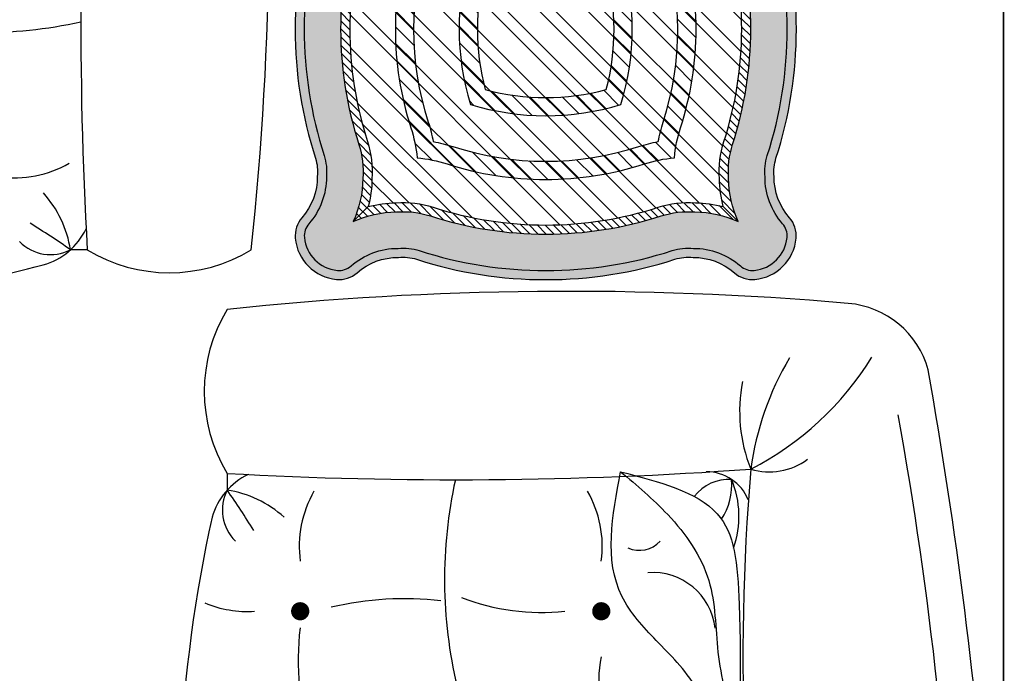
# Model space of a CAD drawing. Units: inches. Extents: x 844 to 2234, y 346 to 1084.
# Tile 41 of 93: x 1266.41 to 1283.63, y 707.78 to 719.22. Entities that reach past the tile are written whole.
import ezdxf

# ---------------------------------------------------------------- set-up
doc = ezdxf.new("R2010")
doc.units = ezdxf.units.IN
doc.header["$MEASUREMENT"] = 0
doc.layers.add('A-WALL', color=7, linetype='Continuous', lineweight=35)
doc.layers.add('furniture', color=8, linetype='Continuous', lineweight=18)
for name, color, linetype in [('RA-AP-01$0$FURN', 3, 'Continuous'), ('RA-AP-01$0$steel', 193, 'Continuous'), ('RA-AP-01$0$WOOD', 64, 'Continuous')]:
    doc.layers.add(name, color=color, linetype=linetype)
pattern_1 = [(45, (0, 1.362436106329781), (-0.0088388347648318, 0.0088388347648318), [])]
pattern_2 = [(45, (0, 1.362436106329781), (-0.0044194173824159, 0.0044194173824159), [])]

# ---------------------------------------------------------------- blocks, each defined once
blk = doc.blocks.new('A$C2FCF5309')
at = {"layer": 'RA-AP-01$0$FURN'}
h = blk.add_hatch(dxfattribs=at)
h.set_pattern_fill('ANSI31', color=256, scale=0.1, style=0)
h.set_pattern_definition(pattern_1)
h.paths.add_polyline_path([(5.038683893313746, -5.169250834004607, -0.1583983521602212), (5.038683893312098, -5.373464580902012, 0.0306258898943267), (5.033304057242972, -5.394827569605182, 0.0306258898948892), (5.01194106853941, -5.40020740567441, -0.1028142994996694), (4.878286182323899, -5.414871334512708), (4.863600873530158, -5.43331743520547, 0.1120482678681049), (5.018059823131753, -5.419248541734471, -0.052642197802937), (5.050972078299936, -5.412495590662115, -0.0526421977994963), (5.057725029371615, -5.379583335496025, 0.1583028414702701), (5.057725029372958, -5.163132079409654, -0.052642197806903), (5.050972078299777, -5.130219824239078, -0.0526421977995126), (5.018059823133679, -5.123466873167369, 0.0215995840215353), (4.988903013548211, -5.115372132362452), (4.975007495303644, -5.132826183367946, -0.0289147572844802), (5.011941068537408, -5.142508009226167, 0.0306258898976746), (5.033304057242868, -5.147887845296027, 0.0306258899022411)])
h.paths.add_polyline_path([(4.975007495303645, -5.132826183367946), (4.988903013548211, -5.115372132362452, 0.1362374241599938), (4.801608567045604, -5.12346687316654, -0.0526421978036853), (4.768696311876971, -5.130219824239102, -0.05264219780204), (4.761943360804856, -5.163132079406747, 0.1583028414743723), (4.761943360806116, -5.379583335498449, -0.0526421977955461), (4.768696311877141, -5.412495590662114, -0.0526421978073986), (4.801608567048022, -5.419248541735437, 0.0454484293938888), (4.863600873530158, -5.43331743520547), (4.878286182323899, -5.414871334512708, -0.0546933379798044), (4.80772732164382, -5.40020740567649, 0.030625889903973), (4.786364332934043, -5.394827569605216, 0.0306258898932853), (4.780984496865101, -5.373464580902791, -0.1583983521638281), (4.780984496864308, -5.169250834000963, 0.03062588989692), (4.786364332933943, -5.147887845296004, 0.0306258898946324), (4.807727321637318, -5.142508009226805, -0.1288932573266927)])
h.paths.add_polyline_path([(4.843422214712861, -5.204945727074827, -0.0783685831716868), (4.924134454130224, -5.196727409635105), (4.939146578618322, -5.177870798323143, 0.1012675676854134), (4.827248748758957, -5.188772261120899, 0.1253648873081696), (4.820394258584192, -5.327034652050361), (4.837127701354095, -5.306015906404253, -0.0981593964869636)], flags=17)
h.paths.add_polyline_path([(4.843422214712824, -5.337769687826355, -0.0311091841722656), (4.837127701354095, -5.306015906404253), (4.820394258584193, -5.32703465205036, 0.0247727657431944), (4.827248748758908, -5.353943153780261, 0.0812754385032542), (4.916962478476905, -5.36629034358622), (4.933684093813825, -5.345286454285511, -0.0876255421014372)], flags=17)
h.paths.add_polyline_path([(4.992419641418037, -5.353943153780226, 0.1506053783834298), (4.992419641417933, -5.188772261120954, 0.0485966419124224), (4.939146578618321, -5.177870798323143), (4.924134454130224, -5.196727409635105, -0.0507799419579301), (4.976246175464031, -5.204945727074882, -0.1296645318906876), (4.97624617546411, -5.337769687826316, -0.0415667119298777), (4.933684093813825, -5.345286454285511), (4.916962478476905, -5.36629034358622, 0.0684915676023693)], flags=17)
h = blk.add_hatch(dxfattribs=at)
h.set_pattern_fill('ANSI31', color=256, scale=0.1, style=0)
h.set_pattern_definition(pattern_1)
h.paths.add_polyline_path([(5.038683893313746, -5.169250834004607, -0.1583983521602212), (5.038683893312098, -5.373464580902012, 0.0306258898943267), (5.033304057242972, -5.394827569605182, 0.0306258898948892), (5.01194106853941, -5.40020740567441, -0.1028142994996694), (4.878286182323899, -5.414871334512708), (4.863600873530158, -5.43331743520547, 0.1120482678681049), (5.018059823131753, -5.419248541734471, -0.052642197802937), (5.050972078299936, -5.412495590662115, -0.0526421977994963), (5.057725029371615, -5.379583335496025, 0.1583028414702701), (5.057725029372958, -5.163132079409654, -0.052642197806903), (5.050972078299777, -5.130219824239078, -0.0526421977995126), (5.018059823133679, -5.123466873167369, 0.0215995840215353), (4.988903013548211, -5.115372132362452), (4.975007495303644, -5.132826183367946, -0.0289147572844802), (5.011941068537408, -5.142508009226167, 0.0306258898976746), (5.033304057242868, -5.147887845296027, 0.0306258899022411)])
h.paths.add_polyline_path([(4.975007495303645, -5.132826183367946), (4.988903013548211, -5.115372132362452, 0.1362374241599938), (4.801608567045604, -5.12346687316654, -0.0526421978036853), (4.768696311876971, -5.130219824239102, -0.05264219780204), (4.761943360804856, -5.163132079406747, 0.1583028414743723), (4.761943360806116, -5.379583335498449, -0.0526421977955461), (4.768696311877141, -5.412495590662114, -0.0526421978073986), (4.801608567048022, -5.419248541735437, 0.0454484293938888), (4.863600873530158, -5.43331743520547), (4.878286182323899, -5.414871334512708, -0.0546933379798044), (4.80772732164382, -5.40020740567649, 0.030625889903973), (4.786364332934043, -5.394827569605216, 0.0306258898932853), (4.780984496865101, -5.373464580902791, -0.1583983521638281), (4.780984496864308, -5.169250834000963, 0.03062588989692), (4.786364332933943, -5.147887845296004, 0.0306258898946324), (4.807727321637318, -5.142508009226805, -0.1288932573266927)])
h.paths.add_polyline_path([(4.843422214712861, -5.204945727074827, -0.0783685831716868), (4.924134454130224, -5.196727409635105), (4.939146578618322, -5.177870798323143, 0.1012675676854134), (4.827248748758957, -5.188772261120899, 0.1253648873081696), (4.820394258584192, -5.327034652050361), (4.837127701354095, -5.306015906404253, -0.0981593964869636)], flags=17)
h.paths.add_polyline_path([(4.843422214712824, -5.337769687826355, -0.0311091841722656), (4.837127701354095, -5.306015906404253), (4.820394258584193, -5.32703465205036, 0.0247727657431944), (4.827248748758908, -5.353943153780261, 0.0812754385032542), (4.916962478476905, -5.36629034358622), (4.933684093813825, -5.345286454285511, -0.0876255421014372)], flags=17)
h.paths.add_polyline_path([(4.992419641418037, -5.353943153780226, 0.1506053783834298), (4.992419641417933, -5.188772261120954, 0.0485966419124224), (4.939146578618321, -5.177870798323143), (4.924134454130224, -5.196727409635105, -0.0507799419579301), (4.976246175464031, -5.204945727074882, -0.1296645318906876), (4.97624617546411, -5.337769687826316, -0.0415667119298777), (4.933684093813825, -5.345286454285511), (4.916962478476905, -5.36629034358622, 0.0684915676023693)], flags=17)
at = {"layer": 'RA-AP-01$0$WOOD'}
h = blk.add_hatch(color=256, dxfattribs=at)
edge = h.paths.add_edge_path()
edge.add_arc((4.683001772622394, -5.026441828662609), 0.0299999999999998, 48.77105092035535, 95.25687599427813)
edge.add_arc((4.684834195088484, -5.046357707450686), 0.0499999999998897, 95.25687599443106, 174.7431240064049)
edge.add_arc((4.664918316300367, -5.044525284985046), 0.0300000000000005, 174.7431240062535, 221.2289490796905)
edge.add_arc((4.591236830209155, -5.109094338216345), 0.0679700159630267, -0.5333070513215148, 41.228949079691915, ccw=False)
edge.add_arc((4.609451302807284, -5.114694777173187), 0.0500000000000008, -17.3556839752095, 5.7020707654044145, ccw=False)
edge.add_arc((5.095208119646659, -5.271357707450659), 0.4603971832811796, 162.0683908477609, 197.9316091523306)
edge.add_arc((4.609451302807533, -5.428020637728902), 0.0500000000000006, -5.702070765320514, 17.355683975293914, ccw=False)
edge.add_arc((4.591236830209412, -5.433621076685779), 0.0679700159630261, -41.228949079600625, 0.5333070514128053, ccw=False)
edge.add_arc((4.664918316300727, -5.498190129916959), 0.0299999999999995, 138.7710509204022, 185.256875994324)
edge.add_arc((4.684834195088642, -5.496357707450695), 0.0499999999997451, 185.2568759946742, 264.74312400432)
edge.add_arc((4.683001772622394, -5.516273586238612), 0.03, 264.743124003969, 311.2289490796446)
edge.add_arc((4.747570825853633, -5.589955072329876), 0.0679700159630271, 89.4666929486321, 131.2289490796457, ccw=False)
edge.add_arc((4.753171264810493, -5.57174059973175), 0.0500000000000015, 72.64431602474701, 95.70207076536133, ccw=False)
edge.add_arc((4.909834195088355, -5.085983782892503), 0.4603971832811774, 252.0683908477147, 287.9316091522845)
edge.add_arc((5.06649712536621, -5.57174059973175), 0.0499999999999999, 84.29792923463953, 107.35568397525361, ccw=False)
edge.add_arc((5.072097564323069, -5.589955072329877), 0.0679700159630274, 48.771050920354185, 90.5333070513679, ccw=False)
edge.add_arc((5.136666617554309, -5.516273586238614), 0.0299999999999997, 228.771050920353, 275.2568759942969)
edge.add_arc((5.134834195088338, -5.496357707450417), 0.0499999999999982, 275.2568759942949, 354.7431240057633)
edge.add_arc((5.154750073876535, -5.498190129916372), 0.0299999999999999, 354.7431240057662, 401.2289490796891)
edge.add_arc((5.228431559967749, -5.433621076685074), 0.0679700159630274, 179.4666929486771, 221.2289490796903, ccw=False)
edge.add_arc((5.210217087369615, -5.428020637728227), 0.0499999999999976, 162.6443160247947, 185.7020707654089, ccw=False)
edge.add_arc((4.724460270530244, -5.271357707450757), 0.4603971832811793, 342.0683908477607, 377.9316091523305)
edge.add_arc((5.210217087369368, -5.114694777172509), 0.0500000000000019, 174.2979292346878, 197.355683975302, ccw=False)
edge.add_arc((5.228431559967489, -5.109094338215639), 0.0679700159630279, 138.7710509203993, 180.5333070514128, ccw=False)
edge.add_arc((5.154750073876174, -5.044525284984457), 0.0300000000000001, 318.771050920401, 365.2568759954636)
edge.add_arc((5.13483419508816, -5.046357707450624), 0.0499999999998349, 5.256875995237118, 84.74312400549572)
edge.add_arc((5.136666617554308, -5.026441828662608), 0.0299999999999994, 84.74312400572185, 131.2289490796446)
edge.add_arc((5.072097564323072, -4.952760342571343), 0.0679700159630261, 269.4666929486298, 311.22894907964354, ccw=False)
edge.add_arc((5.066497125366206, -4.97097481516947), 0.0499999999999992, 252.64431602475162, 275.70207076536565, ccw=False)
edge.add_arc((4.909834195088355, -5.456731632008717), 0.4603971832811764, 72.06839084771546, 107.9316091522853)
edge.add_arc((4.753171264810493, -4.970974815169471), 0.0500000000000016, 264.2979292346387, 287.355683975253, ccw=False)
edge.add_arc((4.747570825853633, -4.952760342571346), 0.0679700159630274, 228.7710509203543, 270.5333070513679, ccw=False)
edge = h.paths.add_edge_path(flags=16)
edge.add_arc((4.683001772622395, -5.026441828662608), 0.019999999999999, 48.7710509203555, 95.2568759942793)
edge.add_arc((4.684834195088469, -5.046357707450671), 0.0399999999998731, 95.2568759944489, 174.7431240064248)
edge.add_arc((4.664918316300404, -5.044525284985035), 0.020000000000036, 174.7431240062186, 221.2289490796461)
edge.add_arc((4.591236830209151, -5.109094338216346), 0.0779700159630296, -0.13764630038667747, 41.228949079689585, ccw=False)
edge.add_arc((4.609451302807307, -5.11469477717304), 0.060000000000024, -17.406127045137907, 5.176192161068002, ccw=False)
edge.add_arc((5.09520811964665, -5.271357707450659), 0.4503971832811708, 162.0623235129628, 197.9376764869162)
edge.add_arc((4.609451302807532, -5.428020637728943), 0.0599999999999982, -5.176192160466428, 17.406127046715312, ccw=False)
edge.add_arc((4.591236830209414, -5.433621076685778), 0.0779700159630257, -41.2289490796029, 0.13764630095249686, ccw=False)
edge.add_arc((4.664918316300731, -5.498190129916961), 0.0200000000000047, 138.7710509204103, 185.2568759943212)
edge.add_arc((4.684834195088606, -5.496357707450731), 0.0399999999997066, 185.2568759947174, 264.7431240043665)
edge.add_arc((4.683001772622369, -5.516273586238541), 0.020000000000069, 264.7431240038842, 311.2289490795622)
edge.add_arc((4.747570825853635, -5.589955072329884), 0.0779700159630344, 89.8623536987642, 131.2289490796432, ccw=False)
edge.add_arc((4.753171264810603, -5.571740599731771), 0.0599999999999895, 72.5938729544394, 95.1761921602253, ccw=False)
edge.add_arc((4.909834195088365, -5.085983782892505), 0.4503971832811724, 252.0623235129989, 287.9376764870498)
edge.add_arc((5.066497125366216, -5.571740599731755), 0.0600000000000047, 84.8238078399923, 107.40612704528041, ccw=False)
edge.add_arc((5.072097564322998, -5.589955072329853), 0.077970015963056, 48.771050920303594, 90.13764630126451, ccw=False)
edge.add_arc((5.136666617554307, -5.516273586238622), 0.0199999999999931, 228.771050920344, 275.2568759943037)
edge.add_arc((5.134834195088338, -5.496357707450416), 0.0400000000000004, 275.2568759942928, 354.7431240057607)
edge.add_arc((5.154750073876533, -5.498190129916375), 0.0200000000000037, 354.7431240057783, 401.2289490796939)
edge.add_arc((5.228431559967745, -5.433621076685076), 0.0779700159630239, 179.8623536995147, 221.2289490796908, ccw=False)
edge.add_arc((5.210217087369586, -5.428020637728345), 0.0600000000000054, 162.5938729554486, 185.1761921609759, ccw=False)
edge.add_arc((4.724460270530243, -5.271357707450766), 0.4503971832811826, 342.0623235128896, 377.937676486982)
edge.add_arc((5.210217087369347, -5.114694777172486), 0.0599999999999777, 174.8238078387611, 197.4061270462219, ccw=False)
edge.add_arc((5.228431559967523, -5.109094338215542), 0.0779700159629885, 138.7710509204687, 180.1376463004423, ccw=False)
edge.add_arc((5.154750073876175, -5.044525284984459), 0.0199999999999989, 318.771050920406, 365.2568759954698)
edge.add_arc((5.134834195088138, -5.046357707450646), 0.0399999999998586, 5.256875995208452, 84.74312400546732)
edge.add_arc((5.136666617554292, -5.02644182866256), 0.0199999999999529, 84.74312400577769, 131.2289490797025)
edge.add_arc((5.072097564323069, -4.952760342571338), 0.077970015963032, 269.86235369901414, 311.2289490796421, ccw=False)
edge.add_arc((5.06649712536618, -4.97097481516946), 0.0600000000000007, 252.5938729548277, 275.17619216047467, ccw=False)
edge.add_arc((4.909834195088353, -5.456731632008716), 0.4503971832811739, 72.06232351293887, 107.9376764867365)
edge.add_arc((4.753171264810429, -4.970974815169467), 0.0599999999999991, 264.82380783985815, 287.40612704769893, ccw=False)
edge.add_arc((4.747570825853681, -4.952760342571361), 0.0779700159630467, 228.7710509203206, 270.13764630113724, ccw=False)
h = blk.add_hatch(color=256, dxfattribs=at)
edge = h.paths.add_edge_path()
edge.add_arc((4.683001772622395, -5.026441828662608), 0.019999999999999, 48.7710509203555, 95.2568759942793)
edge.add_arc((4.684834195088469, -5.046357707450671), 0.0399999999998731, 95.2568759944489, 174.7431240064248)
edge.add_arc((4.664918316300404, -5.044525284985035), 0.020000000000036, 174.7431240062186, 221.2289490796461)
edge.add_arc((4.591236830209151, -5.109094338216346), 0.0779700159630296, -0.13764630038667747, 41.228949079689585, ccw=False)
edge.add_arc((4.609451302807307, -5.11469477717304), 0.060000000000024, -17.406127045137907, 5.176192161068002, ccw=False)
edge.add_arc((5.09520811964665, -5.271357707450659), 0.4503971832811708, 162.0623235129628, 197.9376764869162)
edge.add_arc((4.609451302807532, -5.428020637728943), 0.0599999999999982, -5.176192160466428, 17.406127046715312, ccw=False)
edge.add_arc((4.591236830209414, -5.433621076685778), 0.0779700159630257, -41.2289490796029, 0.13764630095249686, ccw=False)
edge.add_arc((4.664918316300731, -5.498190129916961), 0.0200000000000047, 138.7710509204103, 185.2568759943212)
edge.add_arc((4.684834195088606, -5.496357707450731), 0.0399999999997066, 185.2568759947174, 264.7431240043665)
edge.add_arc((4.683001772622369, -5.516273586238541), 0.020000000000069, 264.7431240038842, 311.2289490795622)
edge.add_arc((4.747570825853635, -5.589955072329884), 0.0779700159630344, 89.8623536987642, 131.2289490796432, ccw=False)
edge.add_arc((4.753171264810603, -5.571740599731771), 0.0599999999999895, 72.5938729544394, 95.1761921602253, ccw=False)
edge.add_arc((4.909834195088365, -5.085983782892505), 0.4503971832811724, 252.0623235129989, 287.9376764870498)
edge.add_arc((5.066497125366216, -5.571740599731755), 0.0600000000000047, 84.8238078399923, 107.40612704528041, ccw=False)
edge.add_arc((5.072097564322998, -5.589955072329853), 0.077970015963056, 48.771050920303594, 90.13764630126451, ccw=False)
edge.add_arc((5.136666617554307, -5.516273586238622), 0.0199999999999931, 228.771050920344, 275.2568759943037)
edge.add_arc((5.134834195088338, -5.496357707450416), 0.0400000000000004, 275.2568759942928, 354.7431240057607)
edge.add_arc((5.154750073876533, -5.498190129916375), 0.0200000000000037, 354.7431240057783, 401.2289490796939)
edge.add_arc((5.228431559967745, -5.433621076685076), 0.0779700159630239, 179.8623536995147, 221.2289490796908, ccw=False)
edge.add_arc((5.210217087369586, -5.428020637728345), 0.0600000000000054, 162.5938729554486, 185.1761921609759, ccw=False)
edge.add_arc((4.724460270530243, -5.271357707450766), 0.4503971832811826, 342.0623235128896, 377.937676486982)
edge.add_arc((5.210217087369347, -5.114694777172486), 0.0599999999999777, 174.8238078387611, 197.4061270462219, ccw=False)
edge.add_arc((5.228431559967523, -5.109094338215542), 0.0779700159629885, 138.7710509204687, 180.1376463004423, ccw=False)
edge.add_arc((5.154750073876175, -5.044525284984459), 0.0199999999999989, 318.771050920406, 365.2568759954698)
edge.add_arc((5.134834195088138, -5.046357707450646), 0.0399999999998586, 5.256875995208452, 84.74312400546732)
edge.add_arc((5.136666617554292, -5.02644182866256), 0.0199999999999529, 84.74312400577769, 131.2289490797025)
edge.add_arc((5.072097564323069, -4.952760342571338), 0.077970015963032, 269.86235369901414, 311.2289490796421, ccw=False)
edge.add_arc((5.06649712536618, -4.97097481516946), 0.0600000000000007, 252.5938729548277, 275.17619216047467, ccw=False)
edge.add_arc((4.909834195088353, -5.456731632008716), 0.4503971832811739, 72.06232351293887, 107.9376764867365)
edge.add_arc((4.753171264810429, -4.970974815169467), 0.0599999999999991, 264.82380783985815, 287.40612704769893, ccw=False)
edge.add_arc((4.747570825853681, -4.952760342571361), 0.0779700159630467, 228.7710509203206, 270.13764630113724, ccw=False)
edge = h.paths.add_edge_path(flags=16)
edge.add_arc((4.591236830209151, -5.109094338216348), 0.1179700159630308, 0.7417751874182841, 24.563326950263672, ccw=False)
edge.add_arc((4.609451302807302, -5.114694777173093), 0.100000000000012, -17.52836504564658, 4.087328884225087, ccw=False)
edge.add_arc((5.095208119646651, -5.271357707450657), 0.4103971832811724, 162.0403002448777, 197.9596997550675)
edge.add_arc((4.60945130280753, -5.428020637728918), 0.1000000000000027, -4.087328883827581, 17.528365046291924, ccw=False)
edge.add_arc((4.591236830209414, -5.433621076685779), 0.1179700159630246, 335.43667305041845, 359.2582248129738, ccw=False)
edge.add_arc((4.747570825853596, -5.589955072329891), 0.117970015963042, 90.7417751868461, 114.5633269496104, ccw=False)
edge.add_arc((4.753171264810559, -5.571740599731767), 0.0999999999999976, 72.47163495370341, 94.0873288836737, ccw=False)
edge.add_arc((4.909834195088367, -5.085983782892503), 0.4103971832811735, 252.0403002449999, 287.9596997551833)
edge.add_arc((5.066497125366205, -5.571740599731755), 0.1000000000000057, 85.91267111645209, 107.5283650455624, ccw=False)
edge.add_arc((5.072097564322985, -5.58995507232986), 0.117970015963046, 65.4366730497672, 89.25822481317113, ccw=False)
edge.add_arc((5.22843155996773, -5.433621076684992), 0.1179700159630096, 180.7417751873964, 204.5633269502712, ccw=False)
edge.add_arc((5.210217087369591, -5.428020637728301), 0.0999999999999969, 162.4716349546276, 184.0873288841682, ccw=False)
edge.add_arc((4.724460270530243, -5.271357707450766), 0.4103971832811825, 342.0403002448147, 377.9596997550345)
edge.add_arc((5.210217087369347, -5.114694777172489), 0.0999999999999796, 175.9126711156995, 197.5283650464392, ccw=False)
edge.add_arc((5.228431559967512, -5.109094338215525), 0.1179700159630019, 155.4366730502992, 179.2582248126247, ccw=False)
edge.add_arc((5.072097564323172, -4.952760342571314), 0.1179700159630537, 270.74177518697286, 294.56332694975765, ccw=False)
edge.add_arc((5.066497125366189, -4.970974815169462), 0.1000000000000017, 252.471634954247, 274.0873288838353, ccw=False)
edge.add_arc((4.909834195088353, -5.456731632008716), 0.4103971832811758, 72.04030024486342, 107.9596997549354)
edge.add_arc((4.75317126481046, -4.970974815169467), 0.1000000000000041, 265.91267111635307, 287.5283650466103, ccw=False)
edge.add_arc((4.747570825853629, -4.952760342571342), 0.1179700159630538, 245.43667304992562, 269.2582248131125, ccw=False)
h = blk.add_hatch(dxfattribs=at)
h.set_pattern_fill('ANSI31', color=256, scale=0.05, style=0)
h.set_pattern_definition(pattern_2)
h.paths.add_polyline_path([(5.105336294329346, -5.394854099602528, 0.0940138826956367), (5.100476366643778, -5.435568764288975, 0.0606271852326483), (5.104678567100611, -5.466202079462671, 0.0606271852344644), (5.074045251925975, -5.46199987900586, 0.0940138827021426), (5.033330587236848, -5.466859806692645, -0.1305325492494615), (4.828072633169377, -5.477944178050054), (4.821119726105699, -5.486677669841435, 0.1336226599878005), (5.036379334063467, -5.476383803188216, -0.0945969211935747), (5.073624810952389, -5.471994942692536, -0.1043170707892296), (5.121137550891356, -5.48266106325342, -0.1043170707868944), (5.110471430330457, -5.435148323315565, -0.0945969211952573), (5.114860290825935, -5.397902846425963, 0.1580239521433527), (5.114860290826324, -5.144812568476775, -0.0945969212010491), (5.110471430330247, -5.10756709158498, -0.1043170707844371), (5.121137550890657, -5.060054351648168, -0.104317070786514), (5.073624810952866, -5.070720472208642, -0.0945969211958523), (5.036379334063063, -5.066331611712874, 0.1580239521426795), (4.783289056114906, -5.066331611712465, -0.0945969211985319), (4.746043579224103, -5.070720472208672, -0.1043170707882665), (4.698530839285552, -5.060054351647925, -0.1043170707867205), (4.709196959846443, -5.10756709158571, -0.094596921196788), (4.704808099350826, -5.144812568475902, 0.1580239521433127), (4.704808099350699, -5.397902846425022, -0.094596921197841), (4.709196959846712, -5.435148323315576, -0.1043170707855109), (4.698530839286393, -5.482661063252921, -0.1043170707864168), (4.746043579224162, -5.471994942692571, -0.0945969211977586), (4.783289056114671, -5.476383803188671, 0.0238966994662183), (4.821119726105699, -5.486677669841435), (4.828072633169378, -5.477944178050054, -0.0269814195959459), (4.786337802940177, -5.466859806692736, 0.0940138827039629), (4.745623138250268, -5.461999879005895, 0.0606271852320776), (4.714989823076826, -5.466202079462476, 0.0606271852304618), (4.719192023533341, -5.435568764289856, 0.0940138826917763), (4.714332095848404, -5.394854099604977, -0.1580706864542086), (4.714332095846561, -5.147861315302034, 0.0940138827032017), (4.719192023533127, -5.107146650612438, 0.0606271852329446), (4.714989823076289, -5.076513335438588, 0.0606271852340035), (4.745623138250698, -5.08071553589536, 0.0940138827025969), (4.786337802940015, -5.075855608208526, -0.1580706864508517), (5.033330587237968, -5.075855608208939, 0.0940138827009578), (5.074045251926627, -5.080715535895319, 0.0606271852322557), (5.104678567100159, -5.076513335438697, 0.0606271852308743), (5.100476366643561, -5.107146650611519, 0.0940138827178109), (5.105336294331983, -5.147861315307182, -0.1580706864490946)])
h = blk.add_hatch(dxfattribs=at)
h.set_pattern_fill('ANSI31', color=256, scale=0.05, style=0)
h.set_pattern_definition(pattern_2)
h.paths.add_polyline_path([(5.105336294329346, -5.394854099602528, 0.0940138826956367), (5.100476366643778, -5.435568764288975, 0.0606271852326483), (5.104678567100611, -5.466202079462671, 0.0606271852344644), (5.074045251925975, -5.46199987900586, 0.0940138827021426), (5.033330587236848, -5.466859806692645, -0.1305325492494615), (4.828072633169377, -5.477944178050054), (4.821119726105699, -5.486677669841435, 0.1336226599878005), (5.036379334063467, -5.476383803188216, -0.0945969211935747), (5.073624810952389, -5.471994942692536, -0.1043170707892296), (5.121137550891356, -5.48266106325342, -0.1043170707868944), (5.110471430330457, -5.435148323315565, -0.0945969211952573), (5.114860290825935, -5.397902846425963, 0.1580239521433527), (5.114860290826324, -5.144812568476775, -0.0945969212010491), (5.110471430330247, -5.10756709158498, -0.1043170707844371), (5.121137550890657, -5.060054351648168, -0.104317070786514), (5.073624810952866, -5.070720472208642, -0.0945969211958523), (5.036379334063063, -5.066331611712874, 0.1580239521426795), (4.783289056114906, -5.066331611712465, -0.0945969211985319), (4.746043579224103, -5.070720472208672, -0.1043170707882665), (4.698530839285552, -5.060054351647925, -0.1043170707867205), (4.709196959846443, -5.10756709158571, -0.094596921196788), (4.704808099350826, -5.144812568475902, 0.1580239521433127), (4.704808099350699, -5.397902846425022, -0.094596921197841), (4.709196959846712, -5.435148323315576, -0.1043170707855109), (4.698530839286393, -5.482661063252921, -0.1043170707864168), (4.746043579224162, -5.471994942692571, -0.0945969211977586), (4.783289056114671, -5.476383803188671, 0.0238966994662183), (4.821119726105699, -5.486677669841435), (4.828072633169378, -5.477944178050054, -0.0269814195959459), (4.786337802940177, -5.466859806692736, 0.0940138827039629), (4.745623138250268, -5.461999879005895, 0.0606271852320776), (4.714989823076826, -5.466202079462476, 0.0606271852304618), (4.719192023533341, -5.435568764289856, 0.0940138826917763), (4.714332095848404, -5.394854099604977, -0.1580706864542086), (4.714332095846561, -5.147861315302034, 0.0940138827032017), (4.719192023533127, -5.107146650612438, 0.0606271852329446), (4.714989823076289, -5.076513335438588, 0.0606271852340035), (4.745623138250698, -5.08071553589536, 0.0940138827025969), (4.786337802940015, -5.075855608208526, -0.1580706864508517), (5.033330587237968, -5.075855608208939, 0.0940138827009578), (5.074045251926627, -5.080715535895319, 0.0606271852322557), (5.104678567100159, -5.076513335438697, 0.0606271852308743), (5.100476366643561, -5.107146650611519, 0.0940138827178109), (5.105336294331983, -5.147861315307182, -0.1580706864490946)])
h = blk.add_hatch(dxfattribs=at)
h.set_pattern_fill('ANSI32,_I', color=256, scale=0.1, style=2)
h.set_pattern_definition([(45, (0, 0), (-0.0265165042944955, 0.0265165042944955), []), (45, (0.0176776695, 0), (-0.0265165042944955, 0.0265165042944955), [])])
h.paths.add_polyline_path([(4.843422214712824, -5.337769687826354, 0.1296645318905289), (4.97624617546411, -5.337769687826316, 0.1296645318906876), (4.976246175464032, -5.204945727074882, 0.129664531890418), (4.843422214712861, -5.204945727074827, 0.129664531890765)], flags=0)
h.paths.add_polyline_path([(5.039131224122924, -5.170637849998464, -0.0326520429852175), (5.033304057242868, -5.147887845296027, -0.0326520429894721), (5.010554052537512, -5.142060678415043, 0.1561383235202698), (4.809114337641437, -5.142060678414318, -0.0326520429925972), (4.786364332933944, -5.147887845296004, -0.0326520429914489), (4.780537166052582, -5.170637850002729, 0.1561383235189577), (4.780537166052134, -5.37207756489719, -0.0326520429934175), (4.786364332934042, -5.394827569605215, -0.0326520429823496), (4.809114337634529, -5.400654736484653, 0.156138323524066), (5.010554052535268, -5.400654736486903, -0.032652042992888), (5.033304057242972, -5.394827569605183, -0.0326520429928733), (5.039131224124712, -5.372077564897496, 0.1561383235226786)], flags=0)
h.paths.add_polyline_path([(4.992419641418037, -5.353943153780226, -0.1506053783832862), (4.827248748758909, -5.353943153780261, -0.1506053783835069), (4.827248748758957, -5.188772261120899, -0.1506053783831346), (4.992419641417933, -5.188772261120954, -0.1506053783834298)], flags=0)
h.paths.add_polyline_path([(4.976246175464111, -5.337769687826316, -0.1296645318905298), (4.843422214712824, -5.337769687826354, -0.129664531890765), (4.843422214712862, -5.204945727074827, -0.1296645318904162), (4.976246175464031, -5.204945727074882, -0.1296645318906876)], flags=0)
h.paths.add_polyline_path([(5.105721254232479, -5.149054940982025, -0.0968902512052664), (5.100476366643561, -5.107146650611519, -0.0606271852308743), (5.104678567100159, -5.076513335438697, -0.0606271852322574), (5.074045251926626, -5.080715535895319, -0.0968902512197216), (5.032136961550132, -5.075470648304253, 0.1564657949319774), (4.787531428625239, -5.075470648304682, -0.0968902512150626), (4.745623138250699, -5.08071553589536, -0.060627185234009), (4.714989823076288, -5.076513335438587, -0.0606271852329501), (4.719192023533127, -5.10714665061244, -0.0968902512185585), (4.713947135942331, -5.149054940988458, 0.1564657949285579), (4.713947135940853, -5.393660473908259, -0.0968902512319826), (4.71919202353334, -5.435568764289873, -0.0606271852304288), (4.714989823076825, -5.466202079462476, -0.0606271852320811), (4.745623138250269, -5.461999879005895, -0.0968902512162649), (4.787531428625332, -5.467244766596559, 0.1564657949327057), (5.032136961551311, -5.46724476659659, -0.0968902512153659), (5.074045251925975, -5.46199987900586, -0.0606271852344627), (5.10467856710061, -5.466202079462671, -0.0606271852326483), (5.100476366643777, -5.435568764288975, -0.0968902512258216), (5.105721254235559, -5.393660473909953, 0.1564657949340142)])
h.paths.add_polyline_path([(5.057725029371625, -5.379583335495999, 0.0526421977995391), (5.050972078299936, -5.412495590662114, 0.0526421978029782), (5.018059823131728, -5.419248541734479, -0.1583028414681072), (4.801608567048168, -5.419248541735485, 0.0526421978076402), (4.76869631187714, -5.412495590662113, 0.0526421977956189), (4.761943360806101, -5.379583335498404, -0.1583028414743129), (4.761943360804846, -5.163132079406778, 0.0526421978020944), (4.768696311876972, -5.130219824239101, 0.0526421978033651), (4.80160856704541, -5.123466873166602, -0.1583028414716875), (5.018059823133628, -5.123466873167353, 0.0526421977995944), (5.050972078299776, -5.130219824239078, 0.0526421978070423), (5.057725029372986, -5.163132079409739, -0.1583028414701848)], flags=16)
h.paths.add_polyline_path([(5.038683893312112, -5.373464580901968, 0.0306258898943915), (5.033304057242972, -5.394827569605182, 0.0306258898948892), (5.01194106853941, -5.40020740567441, -0.1583983521587032), (4.807727321643864, -5.400207405676503, 0.0306258899040366), (4.786364332934043, -5.394827569605215, 0.0306258898931986), (4.780984496865119, -5.37346458090285, -0.1583983521638542), (4.7809844968643, -5.169250834000989, 0.0306258898969596), (4.786364332933945, -5.147887845296004, 0.0306258898946195), (4.807727321637311, -5.142508009226808, -0.1583983521623412), (5.011941068537318, -5.142508009226139, 0.030625889897807), (5.033304057242868, -5.147887845296028, 0.0306258899020632), (5.038683893313706, -5.169250834004486, -0.1583983521602835)], flags=0)
for p, q in [((4.714989823076289, -5.076513335438588), (4.698530839285552, -5.060054351647925)), ((4.714989823076289, -5.076513335438588), (4.698530839285552, -5.060054351647925)), ((5.104678567100159, -5.076513335438697), (5.121137550890656, -5.060054351648169)), ((5.104678567100159, -5.076513335438697), (5.121137550890656, -5.060054351648169)), ((5.10467856710061, -5.466202079462671), (5.121137550891355, -5.482661063253419)), ((5.10467856710061, -5.466202079462671), (5.121137550891355, -5.482661063253419))]:
    blk.add_line(p, q, dxfattribs=at)
for points in [[(4.702773858784635, -5.003879368495489, 0.2056608120285223), (4.680253138923443, -4.996568010480312, 0.3614336704708569), (4.635044498118043, -5.041776651286372, 0.2056608120263112), (4.642355856133262, -5.064297371147306, -0.1842662638101064), (4.65920390179375, -5.10972699154053, -0.1009492694051416), (4.657174869772992, -5.129609908955028, 0.1577727036674954), (4.657174869773219, -5.41310550594699, -0.1009492694051416), (4.659203901794006, -5.432988423361486, -0.1842662638101064), (4.64235585613359, -5.478418043754737, 0.2056608120285221), (4.635044498118431, -5.500938763615934, 0.3614336704593693), (4.680253138922529, -5.546147404420826, 0.2056608120364936), (4.702773858784635, -5.538836046405732, -0.1842662638101064), (4.748203479177874, -5.52198800074528, -0.1009492694051415), (4.768086396592371, -5.524017032766053, 0.1577727036674954), (5.051581993584332, -5.524017032766055, -0.1009492694051416), (5.071464910998829, -5.521988000745282, -0.1842662638101064), (5.116894531392067, -5.538836046405734, 0.2056608120286145), (5.13941525125327, -5.546147404420911, 0.3614336704683636), (5.184623892058835, -5.500938763615299, 0.2056608120285223), (5.177312534043641, -5.478418043754112, -0.1842662638101063), (5.160464488383153, -5.432988423360887, -0.1009492694051416), (5.162493520403909, -5.41310550594639, 0.1577727036674954), (5.162493520403684, -5.129609908954428, -0.1009492694051416), (5.160464488382894, -5.109726991539933, -0.1842662638101064), (5.17731253404331, -5.064297371146681, 0.2056608120337072), (5.184623892058415, -5.041776651284888, 0.3614336704623863), (5.139415251253259, -4.99656801048031, 0.2056608120285223), (5.116894531392067, -5.003879368495487, -0.1842662638101064), (5.071464910998829, -5.020727414155937, -0.1009492694051416), (5.051581993584332, -5.018698382135166, 0.1577727036674956), (4.768086396592371, -5.018698382135168, -0.1009492694051416), (4.748203479177874, -5.020727414155941, -0.1842662638101064)], [(4.702773858784635, -5.003879368495489, 0.2056608120285223), (4.680253138923443, -4.996568010480312, 0.3614336704708569), (4.635044498118043, -5.041776651286372, 0.2056608120263112), (4.642355856133262, -5.064297371147306, -0.1842662638101064), (4.65920390179375, -5.10972699154053, -0.1009492694051416), (4.657174869772992, -5.129609908955028, 0.1577727036674954), (4.657174869773219, -5.41310550594699, -0.1009492694051416), (4.659203901794006, -5.432988423361486, -0.1842662638101064), (4.64235585613359, -5.478418043754737, 0.2056608120285221), (4.635044498118431, -5.500938763615934, 0.3614336704593693), (4.680253138922529, -5.546147404420826, 0.2056608120364936), (4.702773858784635, -5.538836046405732, -0.1842662638101064), (4.748203479177874, -5.52198800074528, -0.1009492694051415), (4.768086396592371, -5.524017032766053, 0.1577727036674954), (5.051581993584332, -5.524017032766055, -0.1009492694051416), (5.071464910998829, -5.521988000745282, -0.1842662638101064), (5.116894531392067, -5.538836046405734, 0.2056608120286145), (5.13941525125327, -5.546147404420911, 0.3614336704683636), (5.184623892058835, -5.500938763615299, 0.2056608120285223), (5.177312534043641, -5.478418043754112, -0.1842662638101063), (5.160464488383153, -5.432988423360887, -0.1009492694051416), (5.162493520403909, -5.41310550594639, 0.1577727036674954), (5.162493520403684, -5.129609908954428, -0.1009492694051416), (5.160464488382894, -5.109726991539933, -0.1842662638101064), (5.17731253404331, -5.064297371146681, 0.2056608120337072), (5.184623892058415, -5.041776651284888, 0.3614336704623863), (5.139415251253259, -4.99656801048031, 0.2056608120285223), (5.116894531392067, -5.003879368495487, -0.1842662638101064), (5.071464910998829, -5.020727414155937, -0.1009492694051416), (5.051581993584332, -5.018698382135166, 0.1577727036674956), (4.768086396592371, -5.018698382135168, -0.1009492694051416), (4.748203479177874, -5.020727414155941, -0.1842662638101064)], [(4.696183163397222, -5.011400188551196, 0.2056608120285295), (4.681169350156427, -5.006525949874411, 0.3614336704708588), (4.645002437512154, -5.042692862519237, 0.2056608120262659), (4.649876676188964, -5.057706675759887, -0.182481815856965), (4.669206621172843, -5.109281651732388, -0.0988540857970112), (4.666703803477437, -5.13264334722805, 0.1578269695851905), (4.666703803477144, -5.410072067672365, -0.0988540858013112), (4.6692066211731, -5.433433763168966, -0.1824818158591246), (4.649876676189301, -5.485008739142145, 0.2056608120284717), (4.64500243751253, -5.500022552382944, 0.3614336704593821), (4.681169350155757, -5.536189465026749, 0.2056608120365057), (4.696183163397221, -5.531315226350026, -0.1824818158605826), (4.747758139370833, -5.51198528136619, -0.0988540857951607), (4.771119834866025, -5.514488099061806, 0.1578269695856264), (5.04854855531107, -5.514488099061688, -0.0988540857929677), (5.071910250805761, -5.511985281366138, -0.1824818158609529), (5.123485226779481, -5.531315226350027, 0.2056608120286893), (5.138499040020282, -5.536189465026812, 0.3614336704683556), (5.174665952664737, -5.500022552382323, 0.2056608120284882), (5.169791713987938, -5.485008739141532, -0.1824818158574124), (5.150461769004059, -5.4334337631689, -0.0988540857940221), (5.152964586699289, -5.410072067673927, 0.1578269695858123), (5.1529645866996, -5.132643347228565, -0.0988540858025403), (5.150461769003872, -5.109281651731659, -0.1824818158565006), (5.169791713987599, -5.057706675759273, 0.2056608120337192), (5.174665952664335, -5.042692862518078, 0.3614336704623903), (5.138499040020236, -5.006525949874406, 0.2056608120285323), (5.123485226779481, -5.011400188551195, -0.1824818158594503), (5.071910250806212, -5.03073013353503, -0.09885408579455), (5.048548555311143, -5.028227315839558, 0.1578269695844942), (4.771119834867991, -5.028227315838772, -0.0988540858042156), (4.747758139370745, -5.030730133535067, -0.1824818158603032)], [(4.696183163397222, -5.011400188551196, 0.2056608120285295), (4.681169350156427, -5.006525949874411, 0.3614336704708588), (4.645002437512154, -5.042692862519237, 0.2056608120262659), (4.649876676188964, -5.057706675759887, -0.182481815856965), (4.669206621172843, -5.109281651732388, -0.0988540857970112), (4.666703803477437, -5.13264334722805, 0.1578269695851905), (4.666703803477144, -5.410072067672365, -0.0988540858013112), (4.6692066211731, -5.433433763168966, -0.1824818158591246), (4.649876676189301, -5.485008739142145, 0.2056608120284717), (4.64500243751253, -5.500022552382944, 0.3614336704593821), (4.681169350155757, -5.536189465026749, 0.2056608120365057), (4.696183163397221, -5.531315226350026, -0.1824818158605826), (4.747758139370833, -5.51198528136619, -0.0988540857951607), (4.771119834866025, -5.514488099061806, 0.1578269695856264), (5.04854855531107, -5.514488099061688, -0.0988540857929677), (5.071910250805761, -5.511985281366138, -0.1824818158609529), (5.123485226779481, -5.531315226350027, 0.2056608120286893), (5.138499040020282, -5.536189465026812, 0.3614336704683556), (5.174665952664737, -5.500022552382323, 0.2056608120284882), (5.169791713987938, -5.485008739141532, -0.1824818158574124), (5.150461769004059, -5.4334337631689, -0.0988540857940221), (5.152964586699289, -5.410072067673927, 0.1578269695858123), (5.1529645866996, -5.132643347228565, -0.0988540858025403), (5.150461769003872, -5.109281651731659, -0.1824818158565006), (5.169791713987599, -5.057706675759273, 0.2056608120337192), (5.174665952664335, -5.042692862518078, 0.3614336704623903), (5.138499040020236, -5.006525949874406, 0.2056608120285323), (5.123485226779481, -5.011400188551195, -0.1824818158594503), (5.071910250806212, -5.03073013353503, -0.09885408579455), (5.048548555311143, -5.028227315839558, 0.1578269695844942), (4.771119834867991, -5.028227315838772, -0.0988540858042156), (4.747758139370745, -5.030730133535067, -0.1824818158603032)], [(4.698530839285552, -5.060054351647925, -0.1043170707867612), (4.709196959846444, -5.107567091585729, -0.0945969211969405), (4.704808099350802, -5.144812568475978, 0.1580239521432241), (4.704808099350681, -5.397902846424963, -0.0945969211980322), (4.709196959846711, -5.43514832331559, -0.104317070785482), (4.698530839286393, -5.482661063252921, -0.1043170707864036), (4.746043579224155, -5.471994942692571, -0.094596921197375), (4.78328905611452, -5.476383803188623, 0.1580239521431959), (5.036379334063463, -5.476383803188218, -0.0945969211935888), (5.07362481095239, -5.471994942692536, -0.1043170707892253), (5.121137550891355, -5.482661063253419, -0.1043170707868921), (5.110471430330457, -5.435148323315565, -0.0945969211954828), (5.114860290825962, -5.397902846425878, 0.158023952143358), (5.114860290826295, -5.144812568476682, -0.0945969212007617), (5.110471430330247, -5.107567091584995, -0.1043170707844689), (5.121137550890656, -5.060054351648169, -0.1043170707864946), (5.073624810952874, -5.070720472208642, -0.0945969211956941), (5.036379334063131, -5.066331611712896, 0.1580239521426976), (4.783289056114946, -5.066331611712452, -0.0945969211986379), (4.746043579224103, -5.070720472208672, -0.1043170707882684)], [(4.698530839285552, -5.060054351647925, -0.1043170707867612), (4.709196959846444, -5.107567091585729, -0.0945969211969405), (4.704808099350802, -5.144812568475978, 0.1580239521432241), (4.704808099350681, -5.397902846424963, -0.0945969211980322), (4.709196959846711, -5.43514832331559, -0.104317070785482), (4.698530839286393, -5.482661063252921, -0.1043170707864036), (4.746043579224155, -5.471994942692571, -0.094596921197375), (4.78328905611452, -5.476383803188623, 0.1580239521431959), (5.036379334063463, -5.476383803188218, -0.0945969211935888), (5.07362481095239, -5.471994942692536, -0.1043170707892253), (5.121137550891355, -5.482661063253419, -0.1043170707868921), (5.110471430330457, -5.435148323315565, -0.0945969211954828), (5.114860290825962, -5.397902846425878, 0.158023952143358), (5.114860290826295, -5.144812568476682, -0.0945969212007617), (5.110471430330247, -5.107567091584995, -0.1043170707844689), (5.121137550890656, -5.060054351648169, -0.1043170707864946), (5.073624810952874, -5.070720472208642, -0.0945969211956941), (5.036379334063131, -5.066331611712896, 0.1580239521426976), (4.783289056114946, -5.066331611712452, -0.0945969211986379), (4.746043579224103, -5.070720472208672, -0.1043170707882684)], [(4.714989823076289, -5.076513335438588, -0.0606271852329464), (4.719192023533127, -5.107146650612439, -0.0940138827030756), (4.714332095846578, -5.147861315301983, 0.1580706864542707), (4.714332095848417, -5.394854099605018, -0.0940138826916965), (4.719192023533341, -5.435568764289864, -0.0606271852304462), (4.714989823076826, -5.466202079462476, -0.0606271852320585), (4.745623138250258, -5.461999879005895, -0.0940138827037036), (4.786337802940059, -5.466859806692699, 0.1580706864500221), (5.033330587236783, -5.466859806692666, -0.0940138827023111), (5.074045251925979, -5.46199987900586, -0.060627185234454), (5.10467856710061, -5.466202079462671, -0.0606271852326709), (5.100476366643777, -5.435568764288963, -0.0940138826958686), (5.105336294329379, -5.394854099602421, 0.1580706864489859), (5.105336294331999, -5.147861315307237, -0.0940138827179432), (5.100476366643561, -5.107146650611518, -0.0606271852308726), (5.104678567100159, -5.076513335438697, -0.0606271852322592), (5.074045251926625, -5.080715535895319, -0.094013882701022), (5.03333058723794, -5.075855608208931, 0.1580706864508015), (4.786337802940061, -5.075855608208511, -0.0940138827027143), (4.745623138250695, -5.08071553589536, -0.0606271852339983)], [(4.714989823076289, -5.076513335438588, -0.0606271852329464), (4.719192023533127, -5.107146650612439, -0.0940138827030756), (4.714332095846578, -5.147861315301983, 0.1580706864542707), (4.714332095848417, -5.394854099605018, -0.0940138826916965), (4.719192023533341, -5.435568764289864, -0.0606271852304462), (4.714989823076826, -5.466202079462476, -0.0606271852320585), (4.745623138250258, -5.461999879005895, -0.0940138827037036), (4.786337802940059, -5.466859806692699, 0.1580706864500221), (5.033330587236783, -5.466859806692666, -0.0940138827023111), (5.074045251925979, -5.46199987900586, -0.060627185234454), (5.10467856710061, -5.466202079462671, -0.0606271852326709), (5.100476366643777, -5.435568764288963, -0.0940138826958686), (5.105336294329379, -5.394854099602421, 0.1580706864489859), (5.105336294331999, -5.147861315307237, -0.0940138827179432), (5.100476366643561, -5.107146650611518, -0.0606271852308726), (5.104678567100159, -5.076513335438697, -0.0606271852322592), (5.074045251926625, -5.080715535895319, -0.094013882701022), (5.03333058723794, -5.075855608208931, 0.1580706864508015), (4.786337802940061, -5.075855608208511, -0.0940138827027143), (4.745623138250695, -5.08071553589536, -0.0606271852339983)], [(4.768696311876972, -5.130219824239102, -0.0526421978019087), (4.761943360804882, -5.163132079406667, 0.1583028414744761), (4.761943360806133, -5.379583335498504, -0.0526421977954539), (4.76869631187714, -5.412495590662113, -0.0526421978076619), (4.801608567048181, -5.419248541735488, 0.1583028414681522), (5.0180598231318, -5.419248541734456, -0.0526421978028585), (5.050972078299936, -5.412495590662114, -0.0526421977992923), (5.057725029371576, -5.379583335496149, 0.1583028414703719), (5.057725029372956, -5.163132079409646, -0.0526421978068888), (5.050972078299776, -5.130219824239078, -0.052642197799403), (5.018059823133745, -5.12346687316739, 0.1583028414717216), (4.801608567045482, -5.123466873166579, -0.0526421978034837)], [(4.768696311876972, -5.130219824239102, -0.0526421978019087), (4.761943360804882, -5.163132079406667, 0.1583028414744761), (4.761943360806133, -5.379583335498504, -0.0526421977954539), (4.76869631187714, -5.412495590662113, -0.0526421978076619), (4.801608567048181, -5.419248541735488, 0.1583028414681522), (5.0180598231318, -5.419248541734456, -0.0526421978028585), (5.050972078299936, -5.412495590662114, -0.0526421977992923), (5.057725029371576, -5.379583335496149, 0.1583028414703719), (5.057725029372956, -5.163132079409646, -0.0526421978068888), (5.050972078299776, -5.130219824239078, -0.052642197799403), (5.018059823133745, -5.12346687316739, 0.1583028414717216), (4.801608567045482, -5.123466873166579, -0.0526421978034837)], [(4.786364332933944, -5.147887845296004, -0.0306258898969254), (4.780984496864308, -5.169250834000966, 0.1583983521638412), (4.780984496865107, -5.373464580902811, -0.0306258898932568), (4.786364332934043, -5.394827569605216, -0.0306258899041339), (4.80772732164393, -5.400207405676526, 0.1583983521586416), (5.011941068539401, -5.400207405674413, -0.0306258898949021), (5.033304057242972, -5.394827569605182, -0.0306258898943513), (5.038683893312104, -5.373464580901996, 0.1583983521602784), (5.038683893313717, -5.16925083400452, -0.0306258899021139), (5.033304057242868, -5.147887845296027, -0.030625889897777), (5.011941068537338, -5.142508009226145, 0.1583983521624288), (4.807727321637224, -5.142508009226835, -0.0306258898944937)], [(4.786364332933944, -5.147887845296004, -0.0306258898969254), (4.780984496864308, -5.169250834000966, 0.1583983521638412), (4.780984496865107, -5.373464580902811, -0.0306258898932568), (4.786364332934043, -5.394827569605216, -0.0306258899041339), (4.80772732164393, -5.400207405676526, 0.1583983521586416), (5.011941068539401, -5.400207405674413, -0.0306258898949021), (5.033304057242972, -5.394827569605182, -0.0306258898943513), (5.038683893312104, -5.373464580901996, 0.1583983521602784), (5.038683893313717, -5.16925083400452, -0.0306258899021139), (5.033304057242868, -5.147887845296027, -0.030625889897777), (5.011941068537338, -5.142508009226145, 0.1583983521624288), (4.807727321637224, -5.142508009226835, -0.0306258898944937)], [(4.827248748758957, -5.1887722611209, 0.1506053783835061), (4.827248748758908, -5.353943153780261, 0.150605378383287), (4.992419641418037, -5.353943153780226, 0.1506053783834298), (4.992419641417933, -5.188772261120954, 0.1506053783831346)], [(4.827248748758957, -5.1887722611209, 0.1506053783835061), (4.827248748758908, -5.353943153780261, 0.150605378383287), (4.992419641418037, -5.353943153780226, 0.1506053783834298), (4.992419641417933, -5.188772261120954, 0.1506053783831346)], [(4.843422214712861, -5.204945727074827, 0.1296645318907659), (4.843422214712824, -5.337769687826355, 0.1296645318905299), (4.976246175464111, -5.337769687826316, 0.1296645318906876), (4.976246175464032, -5.204945727074882, 0.129664531890418)], [(4.843422214712861, -5.204945727074827, 0.1296645318907659), (4.843422214712824, -5.337769687826355, 0.1296645318905299), (4.976246175464111, -5.337769687826316, 0.1296645318906876), (4.976246175464032, -5.204945727074882, 0.129664531890418)]]:
    blk.add_lwpolyline(points, format="xyb", close=True, dxfattribs=at)
blk = doc.blocks.new('A$C7EE91E48')
at = {"layer": 'RA-AP-01$0$FURN'}
blk.add_line((9.775453681024517, -8.916612252413607), (9.757112325609974, -8.91661225241228), dxfattribs=at)
at = {"layer": 'RA-AP-01$0$FURN', "const_width": 0.01}
for points in [[(9.624035873781274, -9.001865189332936, 1), (9.624035873781297, -8.991865189332932, 1)], [(9.624035873780826, -9.322250169057511, -1), (9.624035873780826, -9.332250169057513, -1)]]:
    blk.add_lwpolyline(points, format="xyb", close=True, dxfattribs=at)
at = {"layer": 'RA-AP-01$0$FURN'}
for centre, radius, start, end in [((9.387879261544771, -10.44238280163197), 1.579145581857318, 77.59199468308728, 96.58839125635443), ((9.865453681024029, -9.0661122524033), 0.1744999999876311, 58.95177800404677, 121.0482219959531), ((9.745074433540111, -8.938971204538984), 0.1212957045587361, 157.3375839744822, 183.7314750942433), ((9.706394910853488, -8.972574909806593), 0.0753785023123622, 25.87456190605585, 73.98335472300344), ((9.735181781955493, -8.959417410432842), 0.0479292786975047, 62.80708685435548, 135.4025460716553), ((9.125600268712216, -8.003664990327692), 1.11020813118073, 301.9328608597714, 304.6664773187981), ((9.636732167011939, -8.897645467382876), 0.1218651776285568, 318.0375529564433, 351.0462320954125), ((14.24233490628227, -9.167687782925107), 4.473931917517753, 176.7828902523826, 184.1477233631118), ((6.42249118116022, -9.291612252417751), 3.552808610866049, 355.0473312316413, 6.058872375658039), ((9.56961973833057, -9.296929112294796), 0.3023568492824586, 83.09448255116675, 107.588060785551), ((9.695285873781074, -9.11718462924615), 0.1214118203512435, 60.14190744855965, 97.69166328915595), ((9.286001211781066, -9.111007490545871), 0.3517162425384579, 353.4124896676112, 13.16745705655713), ((9.65905457432348, -9.665283690153952), 0.5100538472773755, 77.61824893593078, 103.3122231353938), ((9.866927508269418, -9.261753835450415), 0.2442261434243043, 158.9017070735605, 185.9923925191661), ((9.695285873780948, -9.206930729144496), 0.1214118203512435, 262.3083367106845, 299.8580925512809), ((9.547087767231618, -9.453923781794167), 0.1295083186917369, 77.99013392028127, 121.3796151021958), ((9.721962050880482, -9.369186052387374), 0.0310151388417235, 155.7760318513891, 227.3789451550393), ((9.597674721851437, -9.383696092249494), 0.0689028341546707, 276.4195171090914, 4.461572645688697), ((9.721016980434092, -9.467332461384675), 0.0478550828899777, 356.575295631534, 52.68338292382147), ((9.727193091302688, -9.442442658911482), 0.05, 292.5826724246039, 359.9999999990535), ((9.76257267867739, -9.40215366480788), 0.0683206773889159, 236.6729861493448, 275.2183950426369), ((9.728288059321612, -9.374174170762846), 0.1042084262671507, 250.4828318717156, 292.8692939327817), ((9.57476488929157, -11.93482586084473), 2.452160434589619, 85.19614643967464, 99.84577117055878), ((9.843355501572116, -9.648968385188004), 0.1698955038956699, 78.87784313594504, 111.8512383801196), ((9.847560443890684, -9.511725524783945), 0.0704710051510922, 163.1338634205325, 216.4126496157095), ((9.736702898899553, -9.812515797398348), 0.3241573581843151, 59.29856748426889, 82.3026350986056), ((10.0808517727553, -9.33652322886128), 0.3382138395168437, 207.2303327094028, 238.2563708342648), ((9.862408234899569, -9.589702786759155), 0.1, 285.499494600857, 355.0473312316416), ((9.079565375949262, -5.436149540861864), 4.284827979137255, 272.1916353285572, 280.2199257473579), ((8.936022170067632, -4.284064429245874), 5.485438776325237, 268.8504034693488, 280.0060732220913)]:
    blk.add_arc(centre, radius, start, end, dxfattribs=at)
for points, knots in [([(9.777267912908336, -9.348473919394923), (9.72881227229245, -9.339303204541801), (9.658611784301481, -9.326017059735285), (9.588175161652856, -9.390102169424527), (9.54880260620782, -9.431527358661508), (9.430932710956684, -9.481194893850247), (9.632509618052595, -9.481144249541359), (9.745531325142556, -9.470177725074079), (9.766284889927373, -9.39059173320999), (9.777267912908336, -9.348473919394923)], [0, 0, 0, 0, 0.1367586589314793, 0.1981301758052369, 0.2677729570689282, 0.3281194902553322, 0.4737578340741565, 0.5765194025309516, 0.692033228742226, 0.692033228742226, 0.692033228742226, 0.692033228742226]), ([(9.777267912908336, -9.348473919394923), (9.762308671078125, -9.366257458082648), (9.729176734078989, -9.405644687068653), (9.66202804490802, -9.45323209587751), (9.577043610038041, -9.451871670355906), (9.52447597485284, -9.465284086012414), (9.497548572726195, -9.472154501784399)], [0, 0, 0, 0, 0.0700185406710175, 0.1550780383534523, 0.2344491945777067, 0.3178048737568313, 0.3178048737568313, 0.3178048737568313, 0.3178048737568313])]:
    blk.add_open_spline(points, degree=3, knots=knots, dxfattribs=at)
blk = doc.blocks.new('A$C7F4351E2')
at = {"layer": 'RA-AP-01$0$FURN'}
blk.add_line((8.352559572600457, -8.927748273106442), (8.35255957259913, -8.909406917691898), dxfattribs=at)
for centre, radius, start, end in [((9.82633505008426, -8.495018853398156), 1.539060359583382, 183.7562265681581, 194.4661216781742), ((9.101231010340802, -8.811349166405407), 0.5100538472773755, 166.6877768646062, 192.3817510640693), ((8.553131949433, -8.847580465862999), 0.1214118203512435, 172.308336710844, 209.8580925514404), ((8.395364730619693, -8.88747637403742), 0.0479292786975047, 134.5974539283447, 207.1929131456445), ((7.439612310514541, -8.277894860794142), 1.11020813118073, 325.333522681202, 328.0671391402286), ((8.408522229993444, -8.858689502935416), 0.0753785023123622, 196.0166452769965, 244.1254380939442), ((8.333592787569726, -8.789026759093863), 0.1218651776285568, 278.9537679045875, 311.9624470435567), ((8.603635103111959, -13.39462949836419), 4.473931917517753, 85.85227663688822, 93.21710974761734), ((8.50205957259015, -9.017748273105955), 0.1744999999876311, 148.9517780040469, 211.0482219959533), ((8.727559572604601, -5.574785773242145), 3.552808610866049, 263.941127624342, 274.9526687683587)]:
    blk.add_arc(centre, radius, start, end, dxfattribs=at)
blk = doc.blocks.new('A$C5D2F253E')
at = {"layer": 'RA-AP-01$0$steel', "xscale": -1}
blk.add_blockref('A$C2FCF5309', (6.339960502260055, 7.248884637679282), dxfattribs=at)
at = {"layer": 'RA-AP-01$0$WOOD', "xscale": -1, "rotation": 180}
for name, p in [('A$C7EE91E48', (-8.833013809079146, -7.288751725733902)), ('A$C7F4351E2', (-7.164808785335935, -7.45332973198748))]:
    blk.add_blockref(name, p, dxfattribs=at)

msp = doc.modelspace()

# ---------------------------------------------------------------- linework, layer by layer
at = {"layer": 'A-WALL'}
msp.add_line((1283.615947594791, 761.3107742764157), (1283.615947594791, 624.3107742764157), dxfattribs=at)

# ---------------------------------------------------------------- block references
at = {"layer": 'furniture', "xscale": -15.94108302203742, "yscale": 15.94108302203742, "zscale": 15.94108302203742, "rotation": 270}
msp.add_blockref('A$C5D2F253E', (1244.08405109492, 696.2584716700112), dxfattribs=at)

doc.saveas('drawing.dxf')
